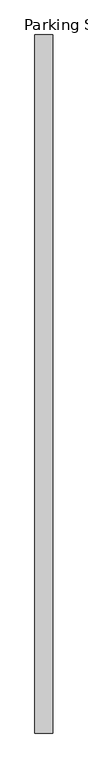
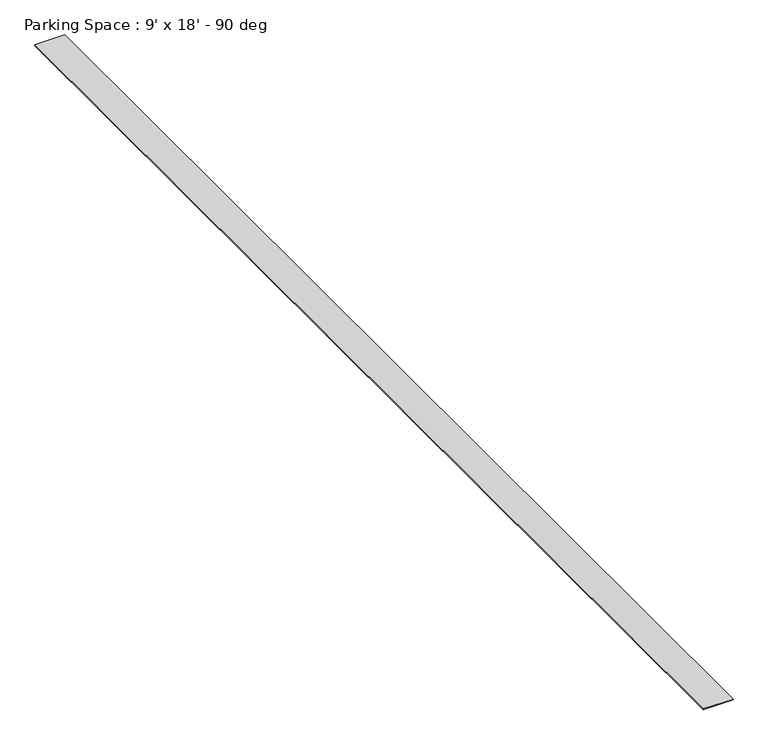
"""IFC4 building model written with IfcOpenShell, lengths in millimetres: proxy geometry, Parking Space : 9' x 18' - 90 deg."""

from ifc_helpers import new_model, si_unit, origin, origin_with_axes, place, context, project, spatial, polyline, outline, extrude, source, transform, mapped, element, save


def parking_space_9_x_18_90_deg_c935943f(model_context):
    return source(origin(), model_context, "Body", "SweptSolid", [
        extrude(outline(polyline([(-50.8, 0.0), (50.8, 0.0), (50.8, -3962.4), (-50.8, -3962.4), (-50.8, 0.0)])), origin_with_axes(), (0.0, 0.0, 1.0), 3.175),
    ])


if __name__ == "__main__":
    model = new_model("IFC4")
    model_context = context("Model", 3, world=origin())
    ifc_project = project(units=[si_unit("LENGTHUNIT", "METRE", prefix="MILLI")], contexts=[model_context])
    site = spatial("IfcSite", under=ifc_project)
    building = spatial("IfcBuilding", under=site)
    placement = place(None, origin())
    parking_space_9_x_18_90_deg_shape = parking_space_9_x_18_90_deg_c935943f(model_context)
    element("IfcBuildingElementProxy", 1, Name="Parking Space : 9' x 18' - 90 deg", ObjectType="Parking Space : 9' x 18' - 90 deg", at=placement, inside=building, context=model_context, shape_type="MappedRepresentation", body=[
        mapped(parking_space_9_x_18_90_deg_shape, transform((0.0, 0.0, 0.0), x_axis=(1.0, 0.0, 0.0), y_axis=(0.0, 1.0, 0.0), z_axis=(0.0, 0.0, 1.0))),
    ])
    save(model, "model.ifc")

# Revit data of these elements
# Type "Parking Space : 9' x 18' - 90 deg"
#   Angle = 90.00°
#   Parking Length = 14' - 0"
#   Parking Width = 5' - 0"
#   pl = 13' - 0"
#   pw = 7' - 0"
# Element 1 (IfcBuildingElementProxy, "Parking Space : 9' x 18' - 90 deg")
#   Materials on its faces: "Parking Stripe"
# Materials
#   "Parking Stripe": class "Paint", colour RGB 250 250 91, transparency 0
